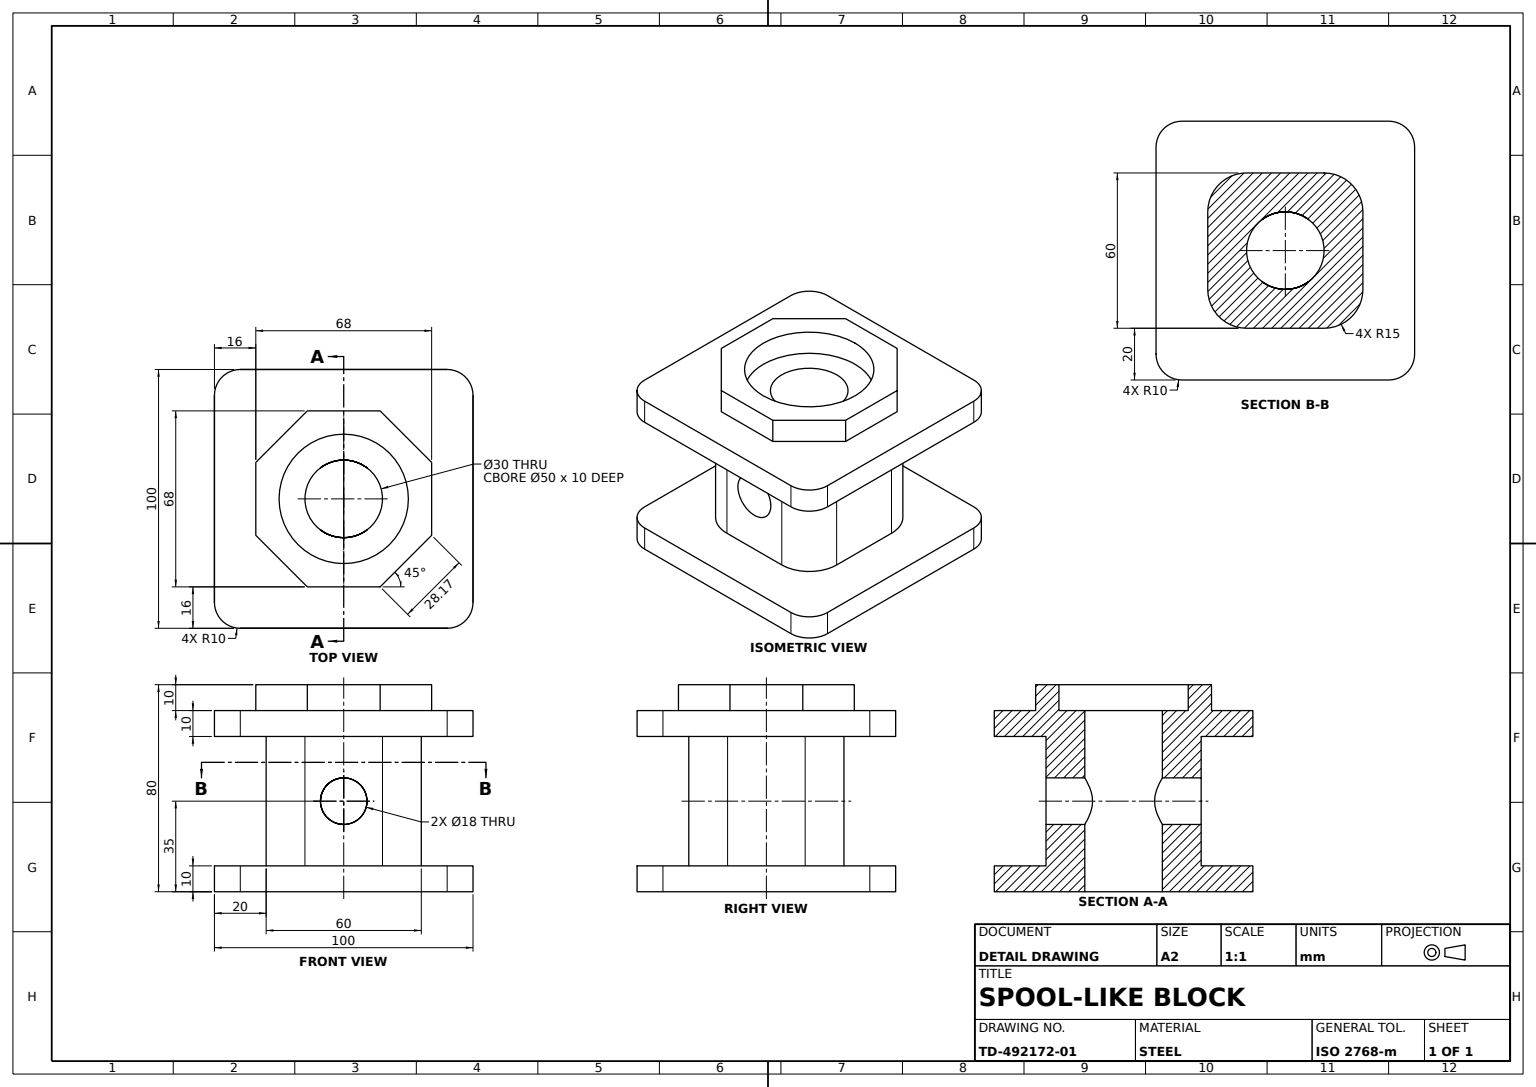
SolidWorks part; units mm, degrees
material "Plain Carbon Steel"
ref_plane "Front Plane" through (0, 0, 0) normal (0, 0, 1) x (1, 0, 0)
ref_plane "Top Plane" through (0, 0, 0) normal (0, 1, 0) x (1, 0, 0)
ref_plane "Right Plane" through (0, 0, 0) normal (1, 0, 0) x (0, 0, -1)
sketch "Base Plate Sketch" plane through (0, 0, 0) normal (0, 1, 0) x (1, 0, 0)
  line L1 (-40, 50) -> (40, 50)
  line L2 (-50, 40) -> (-50, -40)
  line L3 (-40, -50) -> (40, -50)
  line L4 (50, 40) -> (50, -40)
  line L5 (-50, 50) -> (50, -50) construction
  line L6 (-50, -50) -> (50, 50) construction
  circle A0 centre (0, 0) radius 15
  arc A1 (-40, -50) -> (-50, -40) centre (-40, -40) cw
  arc A2 (-40, 50) -> (-50, 40) centre (-40, 40) ccw
  arc A3 (40, 50) -> (50, 40) centre (40, 40) cw
  arc A4 (40, -50) -> (50, -40) centre (40, -40) ccw
  point P0 (0, 0)
  dimension "D3" = 30
  dimension "D4" = 10
  dimension "D1" = 100
  dimension "D2" = 100
extrude "Base Plate" add sketch "Base Plate Sketch" along normal blind 10
sketch "Centre Column Sketch" plane through (0, 10, 0) normal (0, 1, 0) x (1, 0, 0)
  line L1 (-15, 30) -> (15, 30)
  line L2 (-30, 15) -> (-30, -15)
  line L3 (-15, -30) -> (15, -30)
  line L4 (30, 15) -> (30, -15)
  line L5 (-30, 30) -> (30, -30) construction
  line L6 (-30, -30) -> (30, 30) construction
  circle A0 centre (0, 0) radius 15 construction
  circle A1 centre (0, 0) radius 15
  arc A2 (15, -30) -> (30, -15) centre (15, -15) ccw
  arc A3 (15, 30) -> (30, 15) centre (15, 15) cw
  arc A4 (-15, 30) -> (-30, 15) centre (-15, 15) ccw
  arc A5 (-30, -15) -> (-15, -30) centre (-15, -15) ccw
  point P0 (0, 0)
  dimension "D3" = 15
  dimension "D1" = 60
  dimension "D2" = 60
extrude "Centre Column" add sketch "Centre Column Sketch" along normal blind 50
sketch "Top Plate Sketch" plane through (0, 60, 0) normal (0, 1, 0) x (1, 0, 0)
  line L5 (-40, -50) -> (40, -50)
  line L6 (50, -40) -> (50, 40)
  line L7 (40, 50) -> (-40, 50)
  line L12 (-50, 40) -> (-50, -40)
  line L13 (-40, -50) -> (40, -50)
  line L14 (50, -40) -> (50, 40)
  line L15 (40, 50) -> (-40, 50)
  line L16 (-50, 40) -> (-50, -40)
  circle A0 centre (0, 0) radius 15 construction
  circle A1 centre (0, 0) radius 15
  arc A12 (-50, -40) -> (-40, -50) centre (-40, -40) ccw
  arc A13 (40, -50) -> (50, -40) centre (40, -40) ccw
  arc A14 (50, 40) -> (40, 50) centre (40, 40) ccw
  arc A15 (-40, 50) -> (-50, 40) centre (-40, 40) ccw
  arc A16 (-50, -40) -> (-40, -50) centre (-40, -40) ccw
  arc A17 (40, -50) -> (50, -40) centre (40, -40) ccw
  arc A18 (50, 40) -> (40, 50) centre (40, 40) ccw
  arc A19 (-40, 50) -> (-50, 40) centre (-40, 40) ccw
  dimension "D1" = 0
extrude "Top Plate" add sketch "Top Plate Sketch" along normal blind 10
sketch "Octagon Boss Sketch" plane through (0, 70, 0) normal (0, 1, 0) x (1, 0, 0)
  line L1 (34, -14.0833) -> (34, 14.0833)
  line L2 (34, 14.0833) -> (14.0833, 34)
  line L3 (14.0833, 34) -> (-14.0833, 34)
  line L4 (-14.0833, 34) -> (-34, 14.0833)
  line L5 (-34, 14.0833) -> (-34, -14.0833)
  line L6 (-34, -14.0833) -> (-14.0833, -34)
  line L7 (-14.0833, -34) -> (14.0833, -34)
  line L8 (14.0833, -34) -> (34, -14.0833)
  circle A0 centre (0, 0) radius 34 construction
  circle A1 centre (0, 0) radius 25
  dimension "D2" = 50
  dimension "D1" = 68
extrude "Octagon Boss" add sketch "Octagon Boss Sketch" along normal blind 10
hole_wizard "Cross Hole Ø18" positions "Sketch5" profile "Sketch6" hole size "Ø1.0" standard "ANSI Metric" end condition through all
sketch "Sketch5" plane through (0, 0, 30) normal (0, 0, 1) x (1, 0, 0)
  line L0 (-40, 0) -> (40, 0) construction
  point P0 (0, 35)
  dimension "D1" = 35
sketch "Sketch6" plane through (0, 35, 30) normal (1, 0, 0) x (0, -1, 0)
  line L0 (0, 0) -> (0, 80)
  line L1 (0, 80) -> (9, 80)
  line L2 (9, 80) -> (9, 0)
  line L5 (9, 0) -> (0, 0)
  line L11 (0, -6.35) -> (0, 107.95) construction
  dimension "Thru Hole Dia." = 18
  dimension "Thru Hole Depth" = 80
